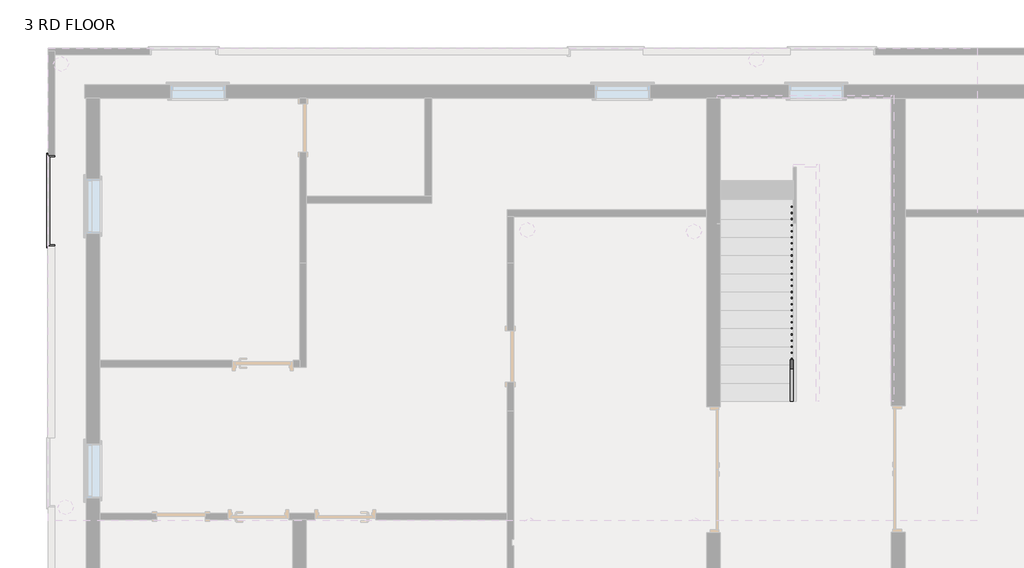
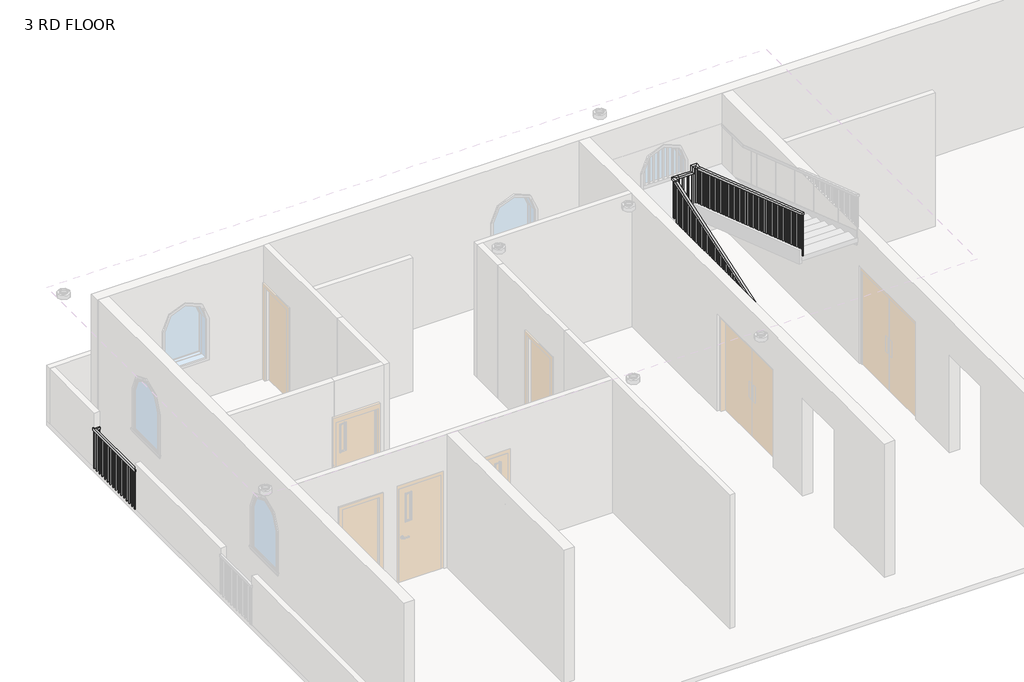
# One storey, part 4 of 7: 2 railings.
"""IFC4 building model written with IfcOpenShell, lengths in millimetres."""

from ifc_helpers import new_model, si_unit, frame, origin, place, context, project, spatial, polyline, outline, extrude, faceted_brep, element, save

model = new_model("IFC4")

# Units and contexts
model_context = context("Model", 3, world=origin())
ifc_project = project(units=[si_unit("LENGTHUNIT", "METRE", prefix="MILLI")], contexts=[model_context])

# Site, building, storey
site = spatial("IfcSite", under=ifc_project)
building = spatial("IfcBuilding", under=site)
storey = spatial("IfcBuildingStorey", under=building, Name="3 RD FLOOR", Elevation=9601.2)

# Railings
placement = place(None, origin())
element("IfcRailing", 1, ObjectType="Handrail - Rectangular", at=placement, inside=storey, context=model_context, shape_type="SolidModel", body=[
    faceted_brep([(-680.3987998, 2564.5067329, 10619.0142857), (-680.3987998, 2564.5067329, 10565.3699957), (-629.5987998, 2564.5067329, 10565.3699957), (-629.5987998, 2564.5067329, 10619.0142857), (-680.3987998, 6450.7067329, 11937.5464286), (-680.3987998, 6501.5067329, 11901.1378529), (-629.5987998, 6501.5067329, 11901.1378529), (-629.5987998, 6450.7067329, 11937.5464286), (-553.3987998, 6577.7067329, 11912.6), (-553.3987998, 6577.7067329, 11963.4), (-273.9987915, 6577.7067329, 11963.4), (-223.1987915, 6577.7067329, 11912.6), (-553.3987998, 6526.9067329, 11912.6), (-223.1987915, 6526.9067329, 11912.6), (-553.3987998, 6526.9067329, 11963.4), (-273.9987915, 6526.9067329, 11963.4), (-146.9987915, 2564.5067329, 13411.2), (-197.7987915, 2564.5067329, 13411.2), (-197.7987915, 2564.5067329, 13357.55571), (-146.9987915, 2564.5067329, 13357.55571), (-146.9987915, 6442.3235624, 12041.8678571), (-146.9987915, 6450.7067329, 12092.6678571), (-197.7987915, 6442.3235624, 12041.8678571), (-197.7987915, 6450.7067329, 12092.6678571), (-680.3987998, 6450.7067329, 11963.4), (-680.3987998, 6501.5067329, 11912.6), (-629.5987998, 6501.5067329, 11912.6), (-629.5987998, 6450.7067329, 11963.4), (-680.3987998, 6577.7067329, 11963.4), (-680.3987998, 6577.7067329, 11912.6), (-629.5987998, 6526.9067329, 11912.6), (-629.5987998, 6526.9067329, 11963.4), (-273.9987915, 6577.7067329, 12092.6678571), (-223.1987915, 6577.7067329, 12041.8678571), (-223.1987915, 6526.9067329, 12041.8678571), (-273.9987915, 6526.9067329, 12092.6678571), (-146.9987915, 6577.7067329, 12092.6678571), (-146.9987915, 6577.7067329, 12041.8678571), (-197.7987915, 6526.9067329, 12041.8678571), (-197.7987915, 6526.9067329, 12092.6678571)], [[[0, 1, 2, 3]], [[1, 0, 4, 5]], [[2, 1, 5, 6]], [[3, 2, 6, 7]], [[0, 3, 7, 4]], [[8, 9, 10, 11]], [[12, 8, 11, 13]], [[14, 12, 13, 15]], [[9, 14, 15, 10]], [[16, 17, 18, 19]], [[20, 21, 16, 19]], [[22, 20, 19, 18]], [[23, 22, 18, 17]], [[21, 23, 17, 16]], [[5, 4, 24, 25]], [[6, 5, 25, 26]], [[7, 6, 26, 27]], [[4, 7, 27, 24]], [[25, 24, 28, 29]], [[26, 25, 29, 30]], [[27, 26, 30, 31]], [[24, 27, 31, 28]], [[29, 28, 9, 8]], [[30, 29, 8, 12]], [[31, 30, 12, 14]], [[28, 31, 14, 9]], [[11, 10, 32, 33]], [[13, 11, 33, 34]], [[15, 13, 34, 35]], [[10, 15, 35, 32]], [[33, 32, 36, 37]], [[34, 33, 37, 38]], [[35, 34, 38, 39]], [[32, 35, 39, 36]], [[37, 36, 21, 20]], [[38, 37, 20, 22]], [[39, 38, 22, 23]], [[36, 39, 23, 21]]]),
    extrude(outline(polyline([(2580.3817329, 13352.1695493), (2599.4317329, 13345.7061565), (2599.4317329, 12393.3857143), (2580.3817329, 12393.3857143), (2580.3817329, 13352.1695493)])), frame((-181.9237915, 0.0, 0.0), z_axis=(1.0, 0.0, 0.0), x_axis=(0.0, 1.0, 0.0)), (0.0, 0.0, 1.0), 19.05),
    extrude(outline(polyline([(2681.9817329, 13317.6981207), (2701.0317329, 13311.2347279), (2701.0317329, 12393.3857143), (2681.9817329, 12393.3857143), (2681.9817329, 13317.6981207)])), frame((-181.9237915, 0.0, 0.0), z_axis=(1.0, 0.0, 0.0), x_axis=(0.0, 1.0, 0.0)), (0.0, 0.0, 1.0), 19.05),
    extrude(outline(polyline([(2783.5817329, 13283.2266922), (2802.6317329, 13276.7632993), (2802.6317329, 12393.3857143), (2783.5817329, 12393.3857143), (2783.5817329, 13283.2266922)])), frame((-181.9237915, 0.0, 0.0), z_axis=(1.0, 0.0, 0.0), x_axis=(0.0, 1.0, 0.0)), (0.0, 0.0, 1.0), 19.05),
    extrude(outline(polyline([(2885.1817329, 13248.7552636), (2904.2317329, 13242.2918707), (2904.2317329, 12289.9714286), (2885.1817329, 12289.9714286), (2885.1817329, 13248.7552636)])), frame((-181.9237915, 0.0, 0.0), z_axis=(1.0, 0.0, 0.0), x_axis=(0.0, 1.0, 0.0)), (0.0, 0.0, 1.0), 19.05),
    extrude(outline(polyline([(2986.7817329, 13214.283835), (3005.8317329, 13207.8204422), (3005.8317329, 12289.9714286), (2986.7817329, 12289.9714286), (2986.7817329, 13214.283835)])), frame((-181.9237915, 0.0, 0.0), z_axis=(1.0, 0.0, 0.0), x_axis=(0.0, 1.0, 0.0)), (0.0, 0.0, 1.0), 19.05),
    extrude(outline(polyline([(3088.3817329, 13179.8124065), (3107.4317329, 13173.3490136), (3107.4317329, 12289.9714286), (3088.3817329, 12289.9714286), (3088.3817329, 13179.8124065)])), frame((-181.9237915, 0.0, 0.0), z_axis=(1.0, 0.0, 0.0), x_axis=(0.0, 1.0, 0.0)), (0.0, 0.0, 1.0), 19.05),
    extrude(outline(polyline([(3189.9817329, 13145.3409779), (3209.0317329, 13138.877585), (3209.0317329, 12186.5571429), (3189.9817329, 12186.5571429), (3189.9817329, 13145.3409779)])), frame((-181.9237915, 0.0, 0.0), z_axis=(1.0, 0.0, 0.0), x_axis=(0.0, 1.0, 0.0)), (0.0, 0.0, 1.0), 19.05),
    extrude(outline(polyline([(3291.5817329, 13110.8695493), (3310.6317329, 13104.4061565), (3310.6317329, 12186.5571429), (3291.5817329, 12186.5571429), (3291.5817329, 13110.8695493)])), frame((-181.9237915, 0.0, 0.0), z_axis=(1.0, 0.0, 0.0), x_axis=(0.0, 1.0, 0.0)), (0.0, 0.0, 1.0), 19.05),
    extrude(outline(polyline([(3393.1817329, 13076.3981207), (3412.2317329, 13069.9347279), (3412.2317329, 12186.5571429), (3393.1817329, 12186.5571429), (3393.1817329, 13076.3981207)])), frame((-181.9237915, 0.0, 0.0), z_axis=(1.0, 0.0, 0.0), x_axis=(0.0, 1.0, 0.0)), (0.0, 0.0, 1.0), 19.05),
    extrude(outline(polyline([(3494.7817329, 13041.9266922), (3513.8317329, 13035.4632993), (3513.8317329, 12083.1428571), (3494.7817329, 12083.1428571), (3494.7817329, 13041.9266922)])), frame((-181.9237915, 0.0, 0.0), z_axis=(1.0, 0.0, 0.0), x_axis=(0.0, 1.0, 0.0)), (0.0, 0.0, 1.0), 19.05),
    extrude(outline(polyline([(3596.3817329, 13007.4552636), (3615.4317329, 13000.9918707), (3615.4317329, 12083.1428571), (3596.3817329, 12083.1428571), (3596.3817329, 13007.4552636)])), frame((-181.9237915, 0.0, 0.0), z_axis=(1.0, 0.0, 0.0), x_axis=(0.0, 1.0, 0.0)), (0.0, 0.0, 1.0), 19.05),
    extrude(outline(polyline([(3697.9817329, 12972.983835), (3717.0317329, 12966.5204422), (3717.0317329, 12083.1428571), (3697.9817329, 12083.1428571), (3697.9817329, 12972.983835)])), frame((-181.9237915, 0.0, 0.0), z_axis=(1.0, 0.0, 0.0), x_axis=(0.0, 1.0, 0.0)), (0.0, 0.0, 1.0), 19.05),
    extrude(outline(polyline([(3799.5817329, 12938.5124065), (3818.6317329, 12932.0490136), (3818.6317329, 11979.7285714), (3799.5817329, 11979.7285714), (3799.5817329, 12938.5124065)])), frame((-181.9237915, 0.0, 0.0), z_axis=(1.0, 0.0, 0.0), x_axis=(0.0, 1.0, 0.0)), (0.0, 0.0, 1.0), 19.05),
    extrude(outline(polyline([(3901.1817329, 12904.0409779), (3920.2317329, 12897.577585), (3920.2317329, 11979.7285714), (3901.1817329, 11979.7285714), (3901.1817329, 12904.0409779)])), frame((-181.9237915, 0.0, 0.0), z_axis=(1.0, 0.0, 0.0), x_axis=(0.0, 1.0, 0.0)), (0.0, 0.0, 1.0), 19.05),
    extrude(outline(polyline([(4002.7817329, 12869.5695493), (4021.8317329, 12863.1061565), (4021.8317329, 11979.7285714), (4002.7817329, 11979.7285714), (4002.7817329, 12869.5695493)])), frame((-181.9237915, 0.0, 0.0), z_axis=(1.0, 0.0, 0.0), x_axis=(0.0, 1.0, 0.0)), (0.0, 0.0, 1.0), 19.05),
    extrude(outline(polyline([(4104.3817329, 12835.0981207), (4123.4317329, 12828.6347279), (4123.4317329, 11876.3142857), (4104.3817329, 11876.3142857), (4104.3817329, 12835.0981207)])), frame((-181.9237915, 0.0, 0.0), z_axis=(1.0, 0.0, 0.0), x_axis=(0.0, 1.0, 0.0)), (0.0, 0.0, 1.0), 19.05),
    extrude(outline(polyline([(4205.9817329, 12800.6266922), (4225.0317329, 12794.1632993), (4225.0317329, 11876.3142857), (4205.9817329, 11876.3142857), (4205.9817329, 12800.6266922)])), frame((-181.9237915, 0.0, 0.0), z_axis=(1.0, 0.0, 0.0), x_axis=(0.0, 1.0, 0.0)), (0.0, 0.0, 1.0), 19.05),
    extrude(outline(polyline([(4307.5817329, 12766.1552636), (4326.6317329, 12759.6918707), (4326.6317329, 11876.3142857), (4307.5817329, 11876.3142857), (4307.5817329, 12766.1552636)])), frame((-181.9237915, 0.0, 0.0), z_axis=(1.0, 0.0, 0.0), x_axis=(0.0, 1.0, 0.0)), (0.0, 0.0, 1.0), 19.05),
    extrude(outline(polyline([(4409.1817329, 12731.683835), (4428.2317329, 12725.2204422), (4428.2317329, 11772.9), (4409.1817329, 11772.9), (4409.1817329, 12731.683835)])), frame((-181.9237915, 0.0, 0.0), z_axis=(1.0, 0.0, 0.0), x_axis=(0.0, 1.0, 0.0)), (0.0, 0.0, 1.0), 19.05),
    extrude(outline(polyline([(4510.7817329, 12697.2124065), (4529.8317329, 12690.7490136), (4529.8317329, 11772.9), (4510.7817329, 11772.9), (4510.7817329, 12697.2124065)])), frame((-181.9237915, 0.0, 0.0), z_axis=(1.0, 0.0, 0.0), x_axis=(0.0, 1.0, 0.0)), (0.0, 0.0, 1.0), 19.05),
    extrude(outline(polyline([(4612.3817329, 12662.7409779), (4631.4317329, 12656.277585), (4631.4317329, 11772.9), (4612.3817329, 11772.9), (4612.3817329, 12662.7409779)])), frame((-181.9237915, 0.0, 0.0), z_axis=(1.0, 0.0, 0.0), x_axis=(0.0, 1.0, 0.0)), (0.0, 0.0, 1.0), 19.05),
    extrude(outline(polyline([(4713.9817329, 12628.2695493), (4733.0317329, 12621.8061565), (4733.0317329, 11669.4857143), (4713.9817329, 11669.4857143), (4713.9817329, 12628.2695493)])), frame((-181.9237915, 0.0, 0.0), z_axis=(1.0, 0.0, 0.0), x_axis=(0.0, 1.0, 0.0)), (0.0, 0.0, 1.0), 19.05),
    extrude(outline(polyline([(4815.5817329, 12593.7981207), (4834.6317329, 12587.3347279), (4834.6317329, 11669.4857143), (4815.5817329, 11669.4857143), (4815.5817329, 12593.7981207)])), frame((-181.9237915, 0.0, 0.0), z_axis=(1.0, 0.0, 0.0), x_axis=(0.0, 1.0, 0.0)), (0.0, 0.0, 1.0), 19.05),
    extrude(outline(polyline([(4917.1817329, 12559.3266922), (4936.2317329, 12552.8632993), (4936.2317329, 11669.4857143), (4917.1817329, 11669.4857143), (4917.1817329, 12559.3266922)])), frame((-181.9237915, 0.0, 0.0), z_axis=(1.0, 0.0, 0.0), x_axis=(0.0, 1.0, 0.0)), (0.0, 0.0, 1.0), 19.05),
    extrude(outline(polyline([(5018.7817329, 12524.8552636), (5037.8317329, 12518.3918707), (5037.8317329, 11566.0714286), (5018.7817329, 11566.0714286), (5018.7817329, 12524.8552636)])), frame((-181.9237915, 0.0, 0.0), z_axis=(1.0, 0.0, 0.0), x_axis=(0.0, 1.0, 0.0)), (0.0, 0.0, 1.0), 19.05),
    extrude(outline(polyline([(5120.3817329, 12490.383835), (5139.4317329, 12483.9204422), (5139.4317329, 11566.0714286), (5120.3817329, 11566.0714286), (5120.3817329, 12490.383835)])), frame((-181.9237915, 0.0, 0.0), z_axis=(1.0, 0.0, 0.0), x_axis=(0.0, 1.0, 0.0)), (0.0, 0.0, 1.0), 19.05),
    extrude(outline(polyline([(5221.9817329, 12455.9124065), (5241.0317329, 12449.4490136), (5241.0317329, 11566.0714286), (5221.9817329, 11566.0714286), (5221.9817329, 12455.9124065)])), frame((-181.9237915, 0.0, 0.0), z_axis=(1.0, 0.0, 0.0), x_axis=(0.0, 1.0, 0.0)), (0.0, 0.0, 1.0), 19.05),
    extrude(outline(polyline([(5323.5817329, 12421.4409779), (5342.6317329, 12414.977585), (5342.6317329, 11462.6571429), (5323.5817329, 11462.6571429), (5323.5817329, 12421.4409779)])), frame((-181.9237915, 0.0, 0.0), z_axis=(1.0, 0.0, 0.0), x_axis=(0.0, 1.0, 0.0)), (0.0, 0.0, 1.0), 19.05),
    extrude(outline(polyline([(5425.1817329, 12386.9695493), (5444.2317329, 12380.5061565), (5444.2317329, 11462.6571429), (5425.1817329, 11462.6571429), (5425.1817329, 12386.9695493)])), frame((-181.9237915, 0.0, 0.0), z_axis=(1.0, 0.0, 0.0), x_axis=(0.0, 1.0, 0.0)), (0.0, 0.0, 1.0), 19.05),
    extrude(outline(polyline([(5526.7817329, 12352.4981207), (5545.8317329, 12346.0347279), (5545.8317329, 11462.6571429), (5526.7817329, 11462.6571429), (5526.7817329, 12352.4981207)])), frame((-181.9237915, 0.0, 0.0), z_axis=(1.0, 0.0, 0.0), x_axis=(0.0, 1.0, 0.0)), (0.0, 0.0, 1.0), 19.05),
    extrude(outline(polyline([(5628.3817329, 12318.0266922), (5647.4317329, 12311.5632993), (5647.4317329, 11359.2428571), (5628.3817329, 11359.2428571), (5628.3817329, 12318.0266922)])), frame((-181.9237915, 0.0, 0.0), z_axis=(1.0, 0.0, 0.0), x_axis=(0.0, 1.0, 0.0)), (0.0, 0.0, 1.0), 19.05),
    extrude(outline(polyline([(5729.9817329, 12283.5552636), (5749.0317329, 12277.0918707), (5749.0317329, 11359.2428571), (5729.9817329, 11359.2428571), (5729.9817329, 12283.5552636)])), frame((-181.9237915, 0.0, 0.0), z_axis=(1.0, 0.0, 0.0), x_axis=(0.0, 1.0, 0.0)), (0.0, 0.0, 1.0), 19.05),
    extrude(outline(polyline([(5831.5817329, 12249.083835), (5850.6317329, 12242.6204422), (5850.6317329, 11359.2428571), (5831.5817329, 11359.2428571), (5831.5817329, 12249.083835)])), frame((-181.9237915, 0.0, 0.0), z_axis=(1.0, 0.0, 0.0), x_axis=(0.0, 1.0, 0.0)), (0.0, 0.0, 1.0), 19.05),
    extrude(outline(polyline([(5933.1817329, 12214.6124065), (5952.2317329, 12208.1490136), (5952.2317329, 11255.8285714), (5933.1817329, 11255.8285714), (5933.1817329, 12214.6124065)])), frame((-181.9237915, 0.0, 0.0), z_axis=(1.0, 0.0, 0.0), x_axis=(0.0, 1.0, 0.0)), (0.0, 0.0, 1.0), 19.05),
    extrude(outline(polyline([(6034.7817329, 12180.1409779), (6053.8317329, 12173.677585), (6053.8317329, 11255.8285714), (6034.7817329, 11255.8285714), (6034.7817329, 12180.1409779)])), frame((-181.9237915, 0.0, 0.0), z_axis=(1.0, 0.0, 0.0), x_axis=(0.0, 1.0, 0.0)), (0.0, 0.0, 1.0), 19.05),
    extrude(outline(polyline([(6136.3817329, 12145.6695493), (6155.4317329, 12139.2061565), (6155.4317329, 11255.8285714), (6136.3817329, 11255.8285714), (6136.3817329, 12145.6695493)])), frame((-181.9237915, 0.0, 0.0), z_axis=(1.0, 0.0, 0.0), x_axis=(0.0, 1.0, 0.0)), (0.0, 0.0, 1.0), 19.05),
    extrude(outline(polyline([(6237.9817329, 12111.1981207), (6257.0317329, 12104.7347279), (6257.0317329, 11152.4142857), (6237.9817329, 11152.4142857), (6237.9817329, 12111.1981207)])), frame((-181.9237915, 0.0, 0.0), z_axis=(1.0, 0.0, 0.0), x_axis=(0.0, 1.0, 0.0)), (0.0, 0.0, 1.0), 19.05),
    extrude(outline(polyline([(6339.5817329, 12076.7266922), (6358.6317329, 12070.2632993), (6358.6317329, 11152.4142857), (6339.5817329, 11152.4142857), (6339.5817329, 12076.7266922)])), frame((-181.9237915, 0.0, 0.0), z_axis=(1.0, 0.0, 0.0), x_axis=(0.0, 1.0, 0.0)), (0.0, 0.0, 1.0), 19.05),
    extrude(outline(polyline([(6441.1817329, 12042.2552636), (6460.2317329, 12035.7918707), (6460.2317329, 11152.4142857), (6441.1817329, 11152.4142857), (6441.1817329, 12042.2552636)])), frame((-181.9237915, 0.0, 0.0), z_axis=(1.0, 0.0, 0.0), x_axis=(0.0, 1.0, 0.0)), (0.0, 0.0, 1.0), 19.05),
    extrude(outline(polyline([(-258.1237998, 6542.7817329), (-258.1237998, 6561.8317329), (-239.0737998, 6561.8317329), (-239.0737998, 6542.7817329), (-258.1237998, 6542.7817329)])), frame((0.0, 0.0, 11049.0), z_axis=(0.0, 0.0, 1.0), x_axis=(1.0, 0.0, 0.0)), (0.0, 0.0, 1.0), 992.8678571),
    extrude(outline(polyline([(-359.7237998, 6542.7817329), (-359.7237998, 6561.8317329), (-340.6737998, 6561.8317329), (-340.6737998, 6542.7817329), (-359.7237998, 6542.7817329)])), frame((0.0, 0.0, 11049.0), z_axis=(0.0, 0.0, 1.0), x_axis=(1.0, 0.0, 0.0)), (0.0, 0.0, 1.0), 863.6),
    extrude(outline(polyline([(-461.3237998, 6542.7817329), (-461.3237998, 6561.8317329), (-442.2737998, 6561.8317329), (-442.2737998, 6542.7817329), (-461.3237998, 6542.7817329)])), frame((0.0, 0.0, 11049.0), z_axis=(0.0, 0.0, 1.0), x_axis=(1.0, 0.0, 0.0)), (0.0, 0.0, 1.0), 863.6),
    extrude(outline(polyline([(-562.9237998, 6542.7817329), (-562.9237998, 6561.8317329), (-543.8737998, 6561.8317329), (-543.8737998, 6542.7817329), (-562.9237998, 6542.7817329)])), frame((0.0, 0.0, 11049.0), z_axis=(0.0, 0.0, 1.0), x_axis=(1.0, 0.0, 0.0)), (0.0, 0.0, 1.0), 863.6),
    extrude(outline(polyline([(-645.4737998, 6517.3817329), (-664.5237998, 6517.3817329), (-664.5237998, 6536.4317329), (-645.4737998, 6536.4317329), (-645.4737998, 6517.3817329)])), frame((0.0, 0.0, 11049.0), z_axis=(0.0, 0.0, 1.0), x_axis=(1.0, 0.0, 0.0)), (0.0, 0.0, 1.0), 863.6),
    extrude(outline(polyline([(6415.7817329, 11872.052585), (6434.8317329, 11878.5159779), (6434.8317329, 10945.5857143), (6415.7817329, 10945.5857143), (6415.7817329, 11872.052585)])), frame((-664.5237998, 0.0, 0.0), z_axis=(1.0, 0.0, 0.0), x_axis=(0.0, 1.0, 0.0)), (0.0, 0.0, 1.0), 19.05),
    extrude(outline(polyline([(6314.1817329, 11837.5811565), (6333.2317329, 11844.0445493), (6333.2317329, 10945.5857143), (6314.1817329, 10945.5857143), (6314.1817329, 11837.5811565)])), frame((-664.5237998, 0.0, 0.0), z_axis=(1.0, 0.0, 0.0), x_axis=(0.0, 1.0, 0.0)), (0.0, 0.0, 1.0), 19.05),
    extrude(outline(polyline([(6212.5817329, 11803.1097279), (6231.6317329, 11809.5731207), (6231.6317329, 10945.5857143), (6212.5817329, 10945.5857143), (6212.5817329, 11803.1097279)])), frame((-664.5237998, 0.0, 0.0), z_axis=(1.0, 0.0, 0.0), x_axis=(0.0, 1.0, 0.0)), (0.0, 0.0, 1.0), 19.05),
    extrude(outline(polyline([(6110.9817329, 11768.6382993), (6130.0317329, 11775.1016922), (6130.0317329, 10842.1714286), (6110.9817329, 10842.1714286), (6110.9817329, 11768.6382993)])), frame((-664.5237998, 0.0, 0.0), z_axis=(1.0, 0.0, 0.0), x_axis=(0.0, 1.0, 0.0)), (0.0, 0.0, 1.0), 19.05),
    extrude(outline(polyline([(6009.3817329, 11734.1668707), (6028.4317329, 11740.6302636), (6028.4317329, 10842.1714286), (6009.3817329, 10842.1714286), (6009.3817329, 11734.1668707)])), frame((-664.5237998, 0.0, 0.0), z_axis=(1.0, 0.0, 0.0), x_axis=(0.0, 1.0, 0.0)), (0.0, 0.0, 1.0), 19.05),
    extrude(outline(polyline([(5907.7817329, 11699.6954422), (5926.8317329, 11706.158835), (5926.8317329, 10842.1714286), (5907.7817329, 10842.1714286), (5907.7817329, 11699.6954422)])), frame((-664.5237998, 0.0, 0.0), z_axis=(1.0, 0.0, 0.0), x_axis=(0.0, 1.0, 0.0)), (0.0, 0.0, 1.0), 19.05),
    extrude(outline(polyline([(5806.1817329, 11665.2240136), (5825.2317329, 11671.6874065), (5825.2317329, 10738.7571429), (5806.1817329, 10738.7571429), (5806.1817329, 11665.2240136)])), frame((-664.5237998, 0.0, 0.0), z_axis=(1.0, 0.0, 0.0), x_axis=(0.0, 1.0, 0.0)), (0.0, 0.0, 1.0), 19.05),
    extrude(outline(polyline([(5704.5817329, 11630.752585), (5723.6317329, 11637.2159779), (5723.6317329, 10738.7571429), (5704.5817329, 10738.7571429), (5704.5817329, 11630.752585)])), frame((-664.5237998, 0.0, 0.0), z_axis=(1.0, 0.0, 0.0), x_axis=(0.0, 1.0, 0.0)), (0.0, 0.0, 1.0), 19.05),
    extrude(outline(polyline([(5602.9817329, 11596.2811565), (5622.0317329, 11602.7445493), (5622.0317329, 10738.7571429), (5602.9817329, 10738.7571429), (5602.9817329, 11596.2811565)])), frame((-664.5237998, 0.0, 0.0), z_axis=(1.0, 0.0, 0.0), x_axis=(0.0, 1.0, 0.0)), (0.0, 0.0, 1.0), 19.05),
    extrude(outline(polyline([(5501.3817329, 11561.8097279), (5520.4317329, 11568.2731207), (5520.4317329, 10635.3428571), (5501.3817329, 10635.3428571), (5501.3817329, 11561.8097279)])), frame((-664.5237998, 0.0, 0.0), z_axis=(1.0, 0.0, 0.0), x_axis=(0.0, 1.0, 0.0)), (0.0, 0.0, 1.0), 19.05),
    extrude(outline(polyline([(5399.7817329, 11527.3382993), (5418.8317329, 11533.8016922), (5418.8317329, 10635.3428571), (5399.7817329, 10635.3428571), (5399.7817329, 11527.3382993)])), frame((-664.5237998, 0.0, 0.0), z_axis=(1.0, 0.0, 0.0), x_axis=(0.0, 1.0, 0.0)), (0.0, 0.0, 1.0), 19.05),
    extrude(outline(polyline([(5298.1817329, 11492.8668707), (5317.2317329, 11499.3302636), (5317.2317329, 10635.3428571), (5298.1817329, 10635.3428571), (5298.1817329, 11492.8668707)])), frame((-664.5237998, 0.0, 0.0), z_axis=(1.0, 0.0, 0.0), x_axis=(0.0, 1.0, 0.0)), (0.0, 0.0, 1.0), 19.05),
    extrude(outline(polyline([(5196.5817329, 11458.3954422), (5215.6317329, 11464.858835), (5215.6317329, 10531.9285714), (5196.5817329, 10531.9285714), (5196.5817329, 11458.3954422)])), frame((-664.5237998, 0.0, 0.0), z_axis=(1.0, 0.0, 0.0), x_axis=(0.0, 1.0, 0.0)), (0.0, 0.0, 1.0), 19.05),
    extrude(outline(polyline([(5094.9817329, 11423.9240136), (5114.0317329, 11430.3874065), (5114.0317329, 10531.9285714), (5094.9817329, 10531.9285714), (5094.9817329, 11423.9240136)])), frame((-664.5237998, 0.0, 0.0), z_axis=(1.0, 0.0, 0.0), x_axis=(0.0, 1.0, 0.0)), (0.0, 0.0, 1.0), 19.05),
    extrude(outline(polyline([(4993.3817329, 11389.452585), (5012.4317329, 11395.9159779), (5012.4317329, 10531.9285714), (4993.3817329, 10531.9285714), (4993.3817329, 11389.452585)])), frame((-664.5237998, 0.0, 0.0), z_axis=(1.0, 0.0, 0.0), x_axis=(0.0, 1.0, 0.0)), (0.0, 0.0, 1.0), 19.05),
    extrude(outline(polyline([(4891.7817329, 11354.9811565), (4910.8317329, 11361.4445493), (4910.8317329, 10428.5142857), (4891.7817329, 10428.5142857), (4891.7817329, 11354.9811565)])), frame((-664.5237998, 0.0, 0.0), z_axis=(1.0, 0.0, 0.0), x_axis=(0.0, 1.0, 0.0)), (0.0, 0.0, 1.0), 19.05),
    extrude(outline(polyline([(4790.1817329, 11320.5097279), (4809.2317329, 11326.9731207), (4809.2317329, 10428.5142857), (4790.1817329, 10428.5142857), (4790.1817329, 11320.5097279)])), frame((-664.5237998, 0.0, 0.0), z_axis=(1.0, 0.0, 0.0), x_axis=(0.0, 1.0, 0.0)), (0.0, 0.0, 1.0), 19.05),
    extrude(outline(polyline([(4688.5817329, 11286.0382993), (4707.6317329, 11292.5016922), (4707.6317329, 10428.5142857), (4688.5817329, 10428.5142857), (4688.5817329, 11286.0382993)])), frame((-664.5237998, 0.0, 0.0), z_axis=(1.0, 0.0, 0.0), x_axis=(0.0, 1.0, 0.0)), (0.0, 0.0, 1.0), 19.05),
    extrude(outline(polyline([(4586.9817329, 11251.5668707), (4606.0317329, 11258.0302636), (4606.0317329, 10325.1), (4586.9817329, 10325.1), (4586.9817329, 11251.5668707)])), frame((-664.5237998, 0.0, 0.0), z_axis=(1.0, 0.0, 0.0), x_axis=(0.0, 1.0, 0.0)), (0.0, 0.0, 1.0), 19.05),
    extrude(outline(polyline([(4485.3817329, 11217.0954422), (4504.4317329, 11223.558835), (4504.4317329, 10325.1), (4485.3817329, 10325.1), (4485.3817329, 11217.0954422)])), frame((-664.5237998, 0.0, 0.0), z_axis=(1.0, 0.0, 0.0), x_axis=(0.0, 1.0, 0.0)), (0.0, 0.0, 1.0), 19.05),
    extrude(outline(polyline([(4383.7817329, 11182.6240136), (4402.8317329, 11189.0874065), (4402.8317329, 10325.1), (4383.7817329, 10325.1), (4383.7817329, 11182.6240136)])), frame((-664.5237998, 0.0, 0.0), z_axis=(1.0, 0.0, 0.0), x_axis=(0.0, 1.0, 0.0)), (0.0, 0.0, 1.0), 19.05),
    extrude(outline(polyline([(4282.1817329, 11148.152585), (4301.2317329, 11154.6159779), (4301.2317329, 10221.6857143), (4282.1817329, 10221.6857143), (4282.1817329, 11148.152585)])), frame((-664.5237998, 0.0, 0.0), z_axis=(1.0, 0.0, 0.0), x_axis=(0.0, 1.0, 0.0)), (0.0, 0.0, 1.0), 19.05),
    extrude(outline(polyline([(4180.5817329, 11113.6811565), (4199.6317329, 11120.1445493), (4199.6317329, 10221.6857143), (4180.5817329, 10221.6857143), (4180.5817329, 11113.6811565)])), frame((-664.5237998, 0.0, 0.0), z_axis=(1.0, 0.0, 0.0), x_axis=(0.0, 1.0, 0.0)), (0.0, 0.0, 1.0), 19.05),
    extrude(outline(polyline([(4078.9817329, 11079.2097279), (4098.0317329, 11085.6731207), (4098.0317329, 10221.6857143), (4078.9817329, 10221.6857143), (4078.9817329, 11079.2097279)])), frame((-664.5237998, 0.0, 0.0), z_axis=(1.0, 0.0, 0.0), x_axis=(0.0, 1.0, 0.0)), (0.0, 0.0, 1.0), 19.05),
    extrude(outline(polyline([(3977.3817329, 11044.7382993), (3996.4317329, 11051.2016922), (3996.4317329, 10118.2714286), (3977.3817329, 10118.2714286), (3977.3817329, 11044.7382993)])), frame((-664.5237998, 0.0, 0.0), z_axis=(1.0, 0.0, 0.0), x_axis=(0.0, 1.0, 0.0)), (0.0, 0.0, 1.0), 19.05),
    extrude(outline(polyline([(3875.7817329, 11010.2668707), (3894.8317329, 11016.7302636), (3894.8317329, 10118.2714286), (3875.7817329, 10118.2714286), (3875.7817329, 11010.2668707)])), frame((-664.5237998, 0.0, 0.0), z_axis=(1.0, 0.0, 0.0), x_axis=(0.0, 1.0, 0.0)), (0.0, 0.0, 1.0), 19.05),
    extrude(outline(polyline([(3774.1817329, 10975.7954422), (3793.2317329, 10982.258835), (3793.2317329, 10118.2714286), (3774.1817329, 10118.2714286), (3774.1817329, 10975.7954422)])), frame((-664.5237998, 0.0, 0.0), z_axis=(1.0, 0.0, 0.0), x_axis=(0.0, 1.0, 0.0)), (0.0, 0.0, 1.0), 19.05),
    extrude(outline(polyline([(3672.5817329, 10941.3240136), (3691.6317329, 10947.7874065), (3691.6317329, 10014.8571429), (3672.5817329, 10014.8571429), (3672.5817329, 10941.3240136)])), frame((-664.5237998, 0.0, 0.0), z_axis=(1.0, 0.0, 0.0), x_axis=(0.0, 1.0, 0.0)), (0.0, 0.0, 1.0), 19.05),
    extrude(outline(polyline([(3570.9817329, 10906.852585), (3590.0317329, 10913.3159779), (3590.0317329, 10014.8571429), (3570.9817329, 10014.8571429), (3570.9817329, 10906.852585)])), frame((-664.5237998, 0.0, 0.0), z_axis=(1.0, 0.0, 0.0), x_axis=(0.0, 1.0, 0.0)), (0.0, 0.0, 1.0), 19.05),
    extrude(outline(polyline([(3469.3817329, 10872.3811565), (3488.4317329, 10878.8445493), (3488.4317329, 10014.8571429), (3469.3817329, 10014.8571429), (3469.3817329, 10872.3811565)])), frame((-664.5237998, 0.0, 0.0), z_axis=(1.0, 0.0, 0.0), x_axis=(0.0, 1.0, 0.0)), (0.0, 0.0, 1.0), 19.05),
    extrude(outline(polyline([(3367.7817329, 10837.9097279), (3386.8317329, 10844.3731207), (3386.8317329, 9911.4428571), (3367.7817329, 9911.4428571), (3367.7817329, 10837.9097279)])), frame((-664.5237998, 0.0, 0.0), z_axis=(1.0, 0.0, 0.0), x_axis=(0.0, 1.0, 0.0)), (0.0, 0.0, 1.0), 19.05),
    extrude(outline(polyline([(3266.1817329, 10803.4382993), (3285.2317329, 10809.9016922), (3285.2317329, 9911.4428571), (3266.1817329, 9911.4428571), (3266.1817329, 10803.4382993)])), frame((-664.5237998, 0.0, 0.0), z_axis=(1.0, 0.0, 0.0), x_axis=(0.0, 1.0, 0.0)), (0.0, 0.0, 1.0), 19.05),
    extrude(outline(polyline([(3164.5817329, 10768.9668707), (3183.6317329, 10775.4302636), (3183.6317329, 9911.4428571), (3164.5817329, 9911.4428571), (3164.5817329, 10768.9668707)])), frame((-664.5237998, 0.0, 0.0), z_axis=(1.0, 0.0, 0.0), x_axis=(0.0, 1.0, 0.0)), (0.0, 0.0, 1.0), 19.05),
    extrude(outline(polyline([(3062.9817329, 10734.4954422), (3082.0317329, 10740.958835), (3082.0317329, 9808.0285714), (3062.9817329, 9808.0285714), (3062.9817329, 10734.4954422)])), frame((-664.5237998, 0.0, 0.0), z_axis=(1.0, 0.0, 0.0), x_axis=(0.0, 1.0, 0.0)), (0.0, 0.0, 1.0), 19.05),
    extrude(outline(polyline([(2961.3817329, 10700.0240136), (2980.4317329, 10706.4874065), (2980.4317329, 9808.0285714), (2961.3817329, 9808.0285714), (2961.3817329, 10700.0240136)])), frame((-664.5237998, 0.0, 0.0), z_axis=(1.0, 0.0, 0.0), x_axis=(0.0, 1.0, 0.0)), (0.0, 0.0, 1.0), 19.05),
    extrude(outline(polyline([(2859.7817329, 10665.552585), (2878.8317329, 10672.0159779), (2878.8317329, 9808.0285714), (2859.7817329, 9808.0285714), (2859.7817329, 10665.552585)])), frame((-664.5237998, 0.0, 0.0), z_axis=(1.0, 0.0, 0.0), x_axis=(0.0, 1.0, 0.0)), (0.0, 0.0, 1.0), 19.05),
    extrude(outline(polyline([(2758.1817329, 10631.0811565), (2777.2317329, 10637.5445493), (2777.2317329, 9704.6142857), (2758.1817329, 9704.6142857), (2758.1817329, 10631.0811565)])), frame((-664.5237998, 0.0, 0.0), z_axis=(1.0, 0.0, 0.0), x_axis=(0.0, 1.0, 0.0)), (0.0, 0.0, 1.0), 19.05),
    extrude(outline(polyline([(2656.5817329, 10596.6097279), (2675.6317329, 10603.0731207), (2675.6317329, 9704.6142857), (2656.5817329, 9704.6142857), (2656.5817329, 10596.6097279)])), frame((-664.5237998, 0.0, 0.0), z_axis=(1.0, 0.0, 0.0), x_axis=(0.0, 1.0, 0.0)), (0.0, 0.0, 1.0), 19.05),
    extrude(outline(polyline([(-181.9237915, 6542.7817329), (-181.9237915, 6561.8317329), (-162.8737915, 6561.8317329), (-162.8737915, 6542.7817329), (-181.9237915, 6542.7817329)])), frame((0.0, 0.0, 11049.0), z_axis=(0.0, 0.0, 1.0), x_axis=(1.0, 0.0, 0.0)), (0.0, 0.0, 1.0), 992.8678571),
    extrude(outline(polyline([(-645.4737998, 6542.7817329), (-664.5237998, 6542.7817329), (-664.5237998, 6561.8317329), (-645.4737998, 6561.8317329), (-645.4737998, 6542.7817329)])), frame((0.0, 0.0, 11049.0), z_axis=(0.0, 0.0, 1.0), x_axis=(1.0, 0.0, 0.0)), (0.0, 0.0, 1.0), 863.6),
    extrude(outline(polyline([(2564.5067329, 13357.55571), (2583.5567329, 13351.0923172), (2583.5567329, 12393.3857143), (2564.5067329, 12393.3857143), (2564.5067329, 13357.55571)])), frame((-181.9237915, 0.0, 0.0), z_axis=(1.0, 0.0, 0.0), x_axis=(0.0, 1.0, 0.0)), (0.0, 0.0, 1.0), 19.05),
    extrude(outline(polyline([(2564.5067329, 10565.3699957), (2583.5567329, 10571.8333886), (2583.5567329, 9704.6142857), (2564.5067329, 9704.6142857), (2564.5067329, 10565.3699957)])), frame((-664.5237998, 0.0, 0.0), z_axis=(1.0, 0.0, 0.0), x_axis=(0.0, 1.0, 0.0)), (0.0, 0.0, 1.0), 19.05),
])
element("IfcRailing", 2, ObjectType="Handrail - Rectangular", at=placement, inside=storey, context=model_context, shape_type="SolidModel", body=[
    faceted_brep([(-12973.9987925, 6656.8711337, 10515.6), (-12973.9987925, 6656.8711337, 10464.8), (-12973.9987925, 6707.6711337, 10464.8), (-12973.9987925, 6707.6711337, 10515.6), (-13062.8987925, 6656.8711337, 10515.6), (-13062.8987925, 6656.8711337, 10464.8), (-13113.6987925, 6707.6711337, 10464.8), (-13113.6987925, 6707.6711337, 10515.6), (-13062.8987925, 5180.1736362, 10515.6), (-13062.8987925, 5180.1736362, 10464.8), (-13113.6987925, 5129.3736362, 10464.8), (-13113.6987925, 5129.3736362, 10515.6), (-12973.9987925, 5180.1736362, 10515.6), (-12973.9987925, 5129.3736362, 10515.6), (-12973.9987925, 5129.3736362, 10464.8), (-12973.9987925, 5180.1736362, 10464.8)], [[[0, 1, 2, 3]], [[1, 0, 4, 5]], [[2, 1, 5, 6]], [[3, 2, 6, 7]], [[0, 3, 7, 4]], [[5, 4, 8, 9]], [[6, 5, 9, 10]], [[7, 6, 10, 11]], [[4, 7, 11, 8]], [[12, 13, 14, 15]], [[9, 8, 12, 15]], [[10, 9, 15, 14]], [[11, 10, 14, 13]], [[8, 11, 13, 12]]]),
    extrude(outline(polyline([(-12996.2237925, 5145.2486362), (-12996.2237925, 5164.2986362), (-12977.1737925, 5164.2986362), (-12977.1737925, 5145.2486362), (-12996.2237925, 5145.2486362)])), frame((0.0, 0.0, 9601.2), z_axis=(0.0, 0.0, 1.0), x_axis=(1.0, 0.0, 0.0)), (0.0, 0.0, 1.0), 863.6),
    extrude(outline(polyline([(-13097.8237925, 5167.7961337), (-13078.7737925, 5167.7961337), (-13078.7737925, 5148.7461337), (-13097.8237925, 5148.7461337), (-13097.8237925, 5167.7961337)])), frame((0.0, 0.0, 9601.2), z_axis=(0.0, 0.0, 1.0), x_axis=(1.0, 0.0, 0.0)), (0.0, 0.0, 1.0), 863.6),
    extrude(outline(polyline([(-13097.8237925, 5269.3961337), (-13078.7737925, 5269.3961337), (-13078.7737925, 5250.3461337), (-13097.8237925, 5250.3461337), (-13097.8237925, 5269.3961337)])), frame((0.0, 0.0, 9601.2), z_axis=(0.0, 0.0, 1.0), x_axis=(1.0, 0.0, 0.0)), (0.0, 0.0, 1.0), 863.6),
    extrude(outline(polyline([(-13097.8237925, 5370.9961337), (-13078.7737925, 5370.9961337), (-13078.7737925, 5351.9461337), (-13097.8237925, 5351.9461337), (-13097.8237925, 5370.9961337)])), frame((0.0, 0.0, 9601.2), z_axis=(0.0, 0.0, 1.0), x_axis=(1.0, 0.0, 0.0)), (0.0, 0.0, 1.0), 863.6),
    extrude(outline(polyline([(-13097.8237925, 5472.5961337), (-13078.7737925, 5472.5961337), (-13078.7737925, 5453.5461337), (-13097.8237925, 5453.5461337), (-13097.8237925, 5472.5961337)])), frame((0.0, 0.0, 9601.2), z_axis=(0.0, 0.0, 1.0), x_axis=(1.0, 0.0, 0.0)), (0.0, 0.0, 1.0), 863.6),
    extrude(outline(polyline([(-13097.8237925, 5574.1961337), (-13078.7737925, 5574.1961337), (-13078.7737925, 5555.1461337), (-13097.8237925, 5555.1461337), (-13097.8237925, 5574.1961337)])), frame((0.0, 0.0, 9601.2), z_axis=(0.0, 0.0, 1.0), x_axis=(1.0, 0.0, 0.0)), (0.0, 0.0, 1.0), 863.6),
    extrude(outline(polyline([(-13097.8237925, 5675.7961337), (-13078.7737925, 5675.7961337), (-13078.7737925, 5656.7461337), (-13097.8237925, 5656.7461337), (-13097.8237925, 5675.7961337)])), frame((0.0, 0.0, 9601.2), z_axis=(0.0, 0.0, 1.0), x_axis=(1.0, 0.0, 0.0)), (0.0, 0.0, 1.0), 863.6),
    extrude(outline(polyline([(-13097.8237925, 5777.3961337), (-13078.7737925, 5777.3961337), (-13078.7737925, 5758.3461337), (-13097.8237925, 5758.3461337), (-13097.8237925, 5777.3961337)])), frame((0.0, 0.0, 9601.2), z_axis=(0.0, 0.0, 1.0), x_axis=(1.0, 0.0, 0.0)), (0.0, 0.0, 1.0), 863.6),
    extrude(outline(polyline([(-13097.8237925, 5878.9961337), (-13078.7737925, 5878.9961337), (-13078.7737925, 5859.9461337), (-13097.8237925, 5859.9461337), (-13097.8237925, 5878.9961337)])), frame((0.0, 0.0, 9601.2), z_axis=(0.0, 0.0, 1.0), x_axis=(1.0, 0.0, 0.0)), (0.0, 0.0, 1.0), 863.6),
    extrude(outline(polyline([(-13097.8237925, 5980.5961337), (-13078.7737925, 5980.5961337), (-13078.7737925, 5961.5461337), (-13097.8237925, 5961.5461337), (-13097.8237925, 5980.5961337)])), frame((0.0, 0.0, 9601.2), z_axis=(0.0, 0.0, 1.0), x_axis=(1.0, 0.0, 0.0)), (0.0, 0.0, 1.0), 863.6),
    extrude(outline(polyline([(-13097.8237925, 6082.1961337), (-13078.7737925, 6082.1961337), (-13078.7737925, 6063.1461337), (-13097.8237925, 6063.1461337), (-13097.8237925, 6082.1961337)])), frame((0.0, 0.0, 9601.2), z_axis=(0.0, 0.0, 1.0), x_axis=(1.0, 0.0, 0.0)), (0.0, 0.0, 1.0), 863.6),
    extrude(outline(polyline([(-13097.8237925, 6183.7961337), (-13078.7737925, 6183.7961337), (-13078.7737925, 6164.7461337), (-13097.8237925, 6164.7461337), (-13097.8237925, 6183.7961337)])), frame((0.0, 0.0, 9601.2), z_axis=(0.0, 0.0, 1.0), x_axis=(1.0, 0.0, 0.0)), (0.0, 0.0, 1.0), 863.6),
    extrude(outline(polyline([(-13097.8237925, 6285.3961337), (-13078.7737925, 6285.3961337), (-13078.7737925, 6266.3461337), (-13097.8237925, 6266.3461337), (-13097.8237925, 6285.3961337)])), frame((0.0, 0.0, 9601.2), z_axis=(0.0, 0.0, 1.0), x_axis=(1.0, 0.0, 0.0)), (0.0, 0.0, 1.0), 863.6),
    extrude(outline(polyline([(-13097.8237925, 6386.9961337), (-13078.7737925, 6386.9961337), (-13078.7737925, 6367.9461337), (-13097.8237925, 6367.9461337), (-13097.8237925, 6386.9961337)])), frame((0.0, 0.0, 9601.2), z_axis=(0.0, 0.0, 1.0), x_axis=(1.0, 0.0, 0.0)), (0.0, 0.0, 1.0), 863.6),
    extrude(outline(polyline([(-13097.8237925, 6488.5961337), (-13078.7737925, 6488.5961337), (-13078.7737925, 6469.5461337), (-13097.8237925, 6469.5461337), (-13097.8237925, 6488.5961337)])), frame((0.0, 0.0, 9601.2), z_axis=(0.0, 0.0, 1.0), x_axis=(1.0, 0.0, 0.0)), (0.0, 0.0, 1.0), 863.6),
    extrude(outline(polyline([(-13097.8237925, 6590.1961337), (-13078.7737925, 6590.1961337), (-13078.7737925, 6571.1461337), (-13097.8237925, 6571.1461337), (-13097.8237925, 6590.1961337)])), frame((0.0, 0.0, 9601.2), z_axis=(0.0, 0.0, 1.0), x_axis=(1.0, 0.0, 0.0)), (0.0, 0.0, 1.0), 863.6),
    extrude(outline(polyline([(-13066.0737925, 6691.7961337), (-13066.0737925, 6672.7461337), (-13085.1237925, 6672.7461337), (-13085.1237925, 6691.7961337), (-13066.0737925, 6691.7961337)])), frame((0.0, 0.0, 9601.2), z_axis=(0.0, 0.0, 1.0), x_axis=(1.0, 0.0, 0.0)), (0.0, 0.0, 1.0), 863.6),
    extrude(outline(polyline([(-13097.8237925, 5164.2986362), (-13078.7737925, 5164.2986362), (-13078.7737925, 5145.2486362), (-13097.8237925, 5145.2486362), (-13097.8237925, 5164.2986362)])), frame((0.0, 0.0, 9601.2), z_axis=(0.0, 0.0, 1.0), x_axis=(1.0, 0.0, 0.0)), (0.0, 0.0, 1.0), 863.6),
    extrude(outline(polyline([(-13078.7737925, 6691.7961337), (-13078.7737925, 6672.7461337), (-13097.8237925, 6672.7461337), (-13097.8237925, 6691.7961337), (-13078.7737925, 6691.7961337)])), frame((0.0, 0.0, 9601.2), z_axis=(0.0, 0.0, 1.0), x_axis=(1.0, 0.0, 0.0)), (0.0, 0.0, 1.0), 863.6),
    extrude(outline(polyline([(-12993.0487925, 5145.2486362), (-12993.0487925, 5164.2986362), (-12973.9987925, 5164.2986362), (-12973.9987925, 5145.2486362), (-12993.0487925, 5145.2486362)])), frame((0.0, 0.0, 9601.2), z_axis=(0.0, 0.0, 1.0), x_axis=(1.0, 0.0, 0.0)), (0.0, 0.0, 1.0), 863.6),
    extrude(outline(polyline([(-12973.9987925, 6691.7961337), (-12973.9987925, 6672.7461337), (-12993.0487925, 6672.7461337), (-12993.0487925, 6691.7961337), (-12973.9987925, 6691.7961337)])), frame((0.0, 0.0, 9601.2), z_axis=(0.0, 0.0, 1.0), x_axis=(1.0, 0.0, 0.0)), (0.0, 0.0, 1.0), 863.6),
])

save(model, "model.ifc")

# Revit data of these elements
# Type "Handrail - Rectangular"
#   Assembly Code = "C2010400"
#   built-in parameter 1008612 = 0.0416667 (stored number, unit not read)
#   built-in parameter 1008611 = 0.0416667 (stored number, unit not read)
#   built-in parameter 1008609 = 0.333333 (stored number, unit not read)
#   built-in parameter 1008604 = 0.166667 (stored number, unit not read)
#   built-in parameter 1008603 = 0.166667 (stored number, unit not read)
#   Railing Height = 3' - 0"
#   built-in parameter 1008630 = 2
#   built-in parameter 1008610 = 2
#   built-in parameter 1008618 = Baluster - Square : 3/4"
# Elements 1, 2 (IfcRailing, "Handrail - Rectangular")
#   Phase Created = New Construction
